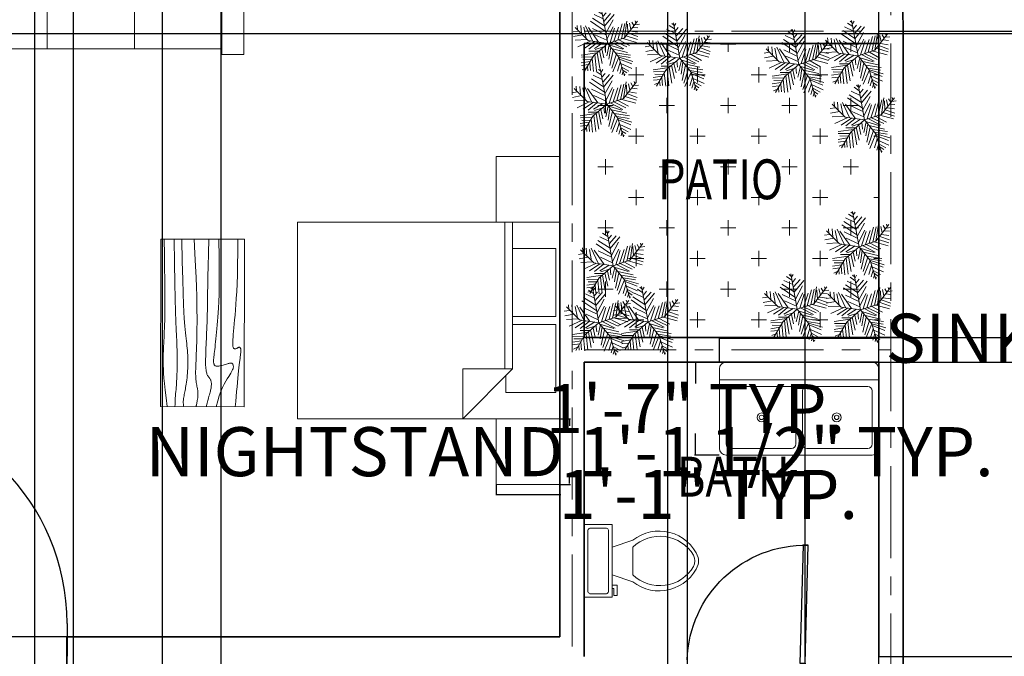
# Model space of a CAD drawing. Units: inches. Extents: x 541 to 1172, y -20 to 887.
# Tile 6 of 8: x 857 to 1058, y 588 to 717. Entities that reach past the tile are written whole.
import ezdxf

# ---------------------------------------------------------------- set-up
doc = ezdxf.new("R2010")
doc.units = ezdxf.units.IN
doc.header["$MEASUREMENT"] = 0
doc.linetypes.add('CENTER', pattern=[50.8, 31.75, -6.35, 6.35, -6.35])
doc.layers.get('0').update_dxf_attribs({"color": 70})
for name, color, linetype, lineweight in [('A-ANNO-DIMS', 2, 'Continuous', 18), ('A-AREA-IDEN', 7, 'Continuous', 20), ('A-DOOR', 4, 'Continuous', 25), ('A-FLOR-FIXT', 9, 'Continuous', 18), ('A-FURN', 30, 'Continuous', 18), ('A-WALL-CNTR', 1, 'CENTER', 13), ('L-PLNT', 70, 'Continuous', 18), ('L-PLNT-PATT', 70, 'Continuous', 13), ('WALL', 7, 'Continuous', 35)]:
    doc.layers.add(name, color=color, linetype=linetype, lineweight=lineweight)
doc.styles.get("Standard").update_dxf_attribs({"font": 'arial.ttf'})
doc.styles.add('YQ_DIM', font='SUPEROS.SHX', dxfattribs={"width": 0.8, "bigfont": 'HZDX.SHX'})
doc.dimstyles.get("Standard").update_dxf_attribs({"dimtxt": 10, "dimasz": 0.18, "dimexe": 0.18, "dimexo": 0.0625, "dimgap": 0.09, "dimtad": 0, "dimtih": 1, "dimtoh": 1, "dimdec": 1, "dimzin": 0, "dimdsep": 46, "dimlunit": 4, "dimtxsty": 'Standard', "dimcen": 0.09, "dimadec": 0, "dimazin": 0, "dimtfac": 1, "dimtdec": 1, "dimtofl": 0, "dimtmove": 0, "dimatfit": 3, "dimfxl": 1, "dimtolj": 1, "dimtzin": 0, "dimarcsym": 0})

# ---------------------------------------------------------------- blocks, each defined once
blk = doc.blocks.new('Sofa - Roundback 7 ft.')
for p, q in [((-12.00002, -32.4421), (-12.00003, -6.5971)), ((11.99997, -32.4421), (11.99998, -6.5971)), ((-36.000027, -34), (-36.000027, -11.4696)), ((-35.999844, -13.3819), (35.9998, -13.3819)), ((35.99998, -34), (35.99998, -11.4696)), ((-36.000027, -32.4421), (35.99998, -32.4421))]:
    blk.add_line(p, q)
for points in [[(-36.000027, -34), (-42.000027, -34), (-42.000027, -8)], [(41.99998, -8), (41.99998, -34), (35.99998, -34)]]:
    blk.add_lwpolyline(points)
for centre, radius, start, end in [((0, -114.25), 114.25, 68.43141, 111.5686), ((-0.00001, -127.1968), 121.1968, 72.72033, 107.2797)]:
    blk.add_arc(centre, radius, start, end)
blk = doc.blocks.new('Bed - Queen')
for p, q in [((0, -80.00003), (0, 0)), ((0, 0), (59.99999, 0)), ((59.99999, 0), (59.99999, -80.00003)), ((7.99999, -1.2), (28.79998, -1.2)), ((7.99999, -14.4), (7.99999, -1.2)), ((28.79998, -1.2), (28.79998, -14.4)), ((31.19999, -1.2), (51.99999, -1.2)), ((31.19999, -14.4), (31.19999, -1.2)), ((51.99999, -1.2), (51.99999, -16.4)), ((0, -14.4), (44.8, -14.4)), ((59.99999, -29.6), (44.8, -14.4)), ((44.8, -14.4), (44.8, -29.6)), ((44.8, -16.8), (0, -16.8)), ((51.99999, -16.4), (46.79936, -16.4)), ((44.8, -29.6), (59.99999, -29.6)), ((59.99999, -80.00003), (0, -80.00003))]:
    blk.add_line(p, q)
blk = doc.blocks.new('Table - Rectangular Woodgrain 60 x 30 in.')
for p, q in [((0, 0), (0, -30)), ((60, 0), (0, 0)), ((60, -30), (60, 0)), ((0, -30), (60, -30))]:
    blk.add_line(p, q)
for points in [[(0, -2.4), (4.8155, -2.418), (9.0302, -2.4688), (12.709, -2.5477), (15.9167, -2.65), (18.7181, -2.7711), (21.1781, -2.9063), (23.3616, -3.0508), (25.3333, -3.2), (27.1477, -3.3495), (28.8172, -3.4958), (30.3437, -3.636), (31.7291, -3.7667), (32.9756, -3.8849), (34.0849, -3.9875), (35.059, -4.0714), (35.9, -4.1334), (36.6114, -4.1711), (37.2041, -4.1854), (37.6906, -4.1779), (38.0833, -4.15), (38.3948, -4.1034), (38.6375, -4.0396), (38.8239, -3.9602), (38.9666, -3.8667), (39.0764, -3.7608), (39.1573, -3.6448), (39.2116, -3.521), (39.2416, -3.3917), (39.2498, -3.2593), (39.2385, -3.1261), (39.21, -2.9944), (39.1666, -2.8667), (39.111, -2.7447), (39.0468, -2.6281), (38.978, -2.5163), (38.9083, -2.4083), (38.8418, -2.3035), (38.7823, -2.201), (38.7337, -2.1001), (38.7, -2), (38.6844, -1.9003), (38.6875, -1.8021), (38.7094, -1.707), (38.75, -1.6167), (38.8094, -1.5326), (38.8875, -1.4563), (38.9844, -1.3893), (39.1, -1.3333), (39.2351, -1.2896), (39.3937, -1.2583), (39.5804, -1.2396), (39.8, -1.2333), (40.057, -1.2396), (40.3562, -1.2583), (40.7023, -1.2896), (41.1, -1.3333), (41.5547, -1.3895), (42.0755, -1.4573), (42.6721, -1.5361), (43.3542, -1.625), (44.1316, -1.7233), (45.014, -1.8302), (46.0114, -1.9449), (47.1333, -2.0667), (48.3862, -2.1947), (49.7625, -2.3281), (51.2513, -2.4663), (52.8416, -2.6083), (54.5226, -2.7535), (56.2833, -2.9011), (58.1127, -3.0501), (60, -3.2)], [(0, -9.2), (6.5759, -9.0858), (11.9385, -9.0365), (16.2527, -9.0418), (19.6833, -9.0917), (22.3952, -9.1759), (24.5531, -9.2844), (26.322, -9.4069), (27.8666, -9.5333), (29.3241, -9.6553), (30.7203, -9.7719), (32.0532, -9.8837), (33.3208, -9.9917), (34.5213, -10.0965), (35.6526, -10.199), (36.7128, -10.2999), (37.7, -10.4), (38.6129, -10.4996), (39.4531, -10.5969), (40.223, -10.6895), (40.925, -10.775), (41.5613, -10.8512), (42.1344, -10.9156), (42.6465, -10.966), (43.1, -11), (43.4976, -11.0158), (43.8437, -11.0136), (44.143, -10.9942), (44.4, -10.9583), (44.6195, -10.9069), (44.8062, -10.8406), (44.9648, -10.7603), (45.1, -10.6667), (45.2155, -10.5598), (45.3114, -10.4365), (45.3871, -10.2929), (45.4416, -10.125), (45.4743, -9.929), (45.4844, -9.7011), (45.4709, -9.4371), (45.4333, -9.1333), (45.3716, -8.7883), (45.2896, -8.4104), (45.1919, -8.0107), (45.0833, -7.6), (44.9685, -7.1893), (44.8521, -6.7896), (44.7388, -6.4117), (44.6333, -6.0667), (44.54, -5.7628), (44.4614, -5.4979), (44.4001, -5.2675), (44.3583, -5.0667), (44.3384, -4.8909), (44.3427, -4.7354), (44.3736, -4.5956), (44.4333, -4.4667), (44.5236, -4.3453), (44.6427, -4.2333), (44.7884, -4.1339), (44.9583, -4.05), (45.1501, -3.9849), (45.3614, -3.9417), (45.59, -3.9234), (45.8333, -3.9333), (46.0915, -3.9749), (46.3734, -4.0531), (46.6906, -4.1736), (47.0542, -4.3417), (47.4756, -4.5629), (47.9661, -4.8427), (48.5372, -5.1866), (49.2, -5.6), (49.9676, -6.0844), (50.8594, -6.625), (51.8965, -7.2031), (53.1, -7.8), (54.491, -8.3969), (56.0906, -8.975), (57.9199, -9.5156), (60, -10)], [(0, -12.8), (5.1847, -12.9322), (9.6213, -13.0323), (13.3963, -13.1059), (16.5958, -13.1583), (19.3063, -13.1952), (21.614, -13.2219), (23.6054, -13.2439), (25.3666, -13.2667), (26.9728, -13.2947), (28.4531, -13.3281), (29.8256, -13.3663), (31.1083, -13.4083), (32.3191, -13.4535), (33.476, -13.501), (34.597, -13.5501), (35.7, -13.6), (36.7984, -13.6497), (37.8875, -13.6979), (38.9578, -13.743), (40, -13.7833), (41.0047, -13.8174), (41.9625, -13.8438), (42.864, -13.8607), (43.7, -13.8667), (44.4631, -13.8604), (45.1552, -13.8417), (45.7801, -13.8104), (46.3416, -13.7667), (46.8439, -13.7104), (47.2906, -13.6417), (47.6858, -13.5604), (48.0333, -13.4667), (48.3375, -13.3608), (48.6042, -13.2448), (48.8396, -13.121), (49.05, -12.9917), (49.2417, -12.8593), (49.4208, -12.7261), (49.5937, -12.5944), (49.7667, -12.4667), (49.9452, -12.3451), (50.1323, -12.2313), (50.3303, -12.1268), (50.5416, -12.0333), (50.7686, -11.9524), (51.0135, -11.8854), (51.2788, -11.8341), (51.5666, -11.8), (51.8785, -11.7843), (52.2116, -11.7865), (52.562, -11.8059), (52.926, -11.8417), (53.2998, -11.8931), (53.6795, -11.9594), (54.0614, -12.0397), (54.4416, -12.1333), (54.8223, -12.2401), (55.2293, -12.3625), (55.6942, -12.5037), (56.2489, -12.6667), (56.9251, -12.8547), (57.7545, -13.0708), (58.7689, -13.3182), (60, -13.6)], [(0, -18), (5.124, -17.7273), (9.6609, -17.5057), (13.6705, -17.3303), (17.2125, -17.1958), (20.3467, -17.0973), (23.1328, -17.0297), (25.6307, -16.9878), (27.9, -16.9667), (29.9928, -16.9617), (31.9302, -16.9703), (33.7254, -16.9907), (35.3917, -17.0208), (36.9423, -17.0588), (38.3906, -17.1026), (39.7499, -17.1503), (41.0333, -17.2), (42.2519, -17.2496), (43.4073, -17.2969), (44.4986, -17.3395), (45.525, -17.375), (46.4858, -17.4012), (47.3802, -17.4156), (48.2074, -17.416), (48.9667, -17.4), (49.6583, -17.3662), (50.2872, -17.3167), (50.8595, -17.2547), (51.3812, -17.1833), (51.8584, -17.1057), (52.2971, -17.025), (52.7034, -16.9443), (53.0833, -16.8667), (53.443, -16.7951), (53.789, -16.7313), (54.128, -16.6768), (54.4666, -16.6334), (54.8115, -16.6024), (55.1693, -16.5854), (55.5465, -16.5841), (55.95, -16.6), (56.3828, -16.6337), (56.8346, -16.6823), (57.2915, -16.7418), (57.7396, -16.8084), (58.165, -16.878), (58.5539, -16.9469), (58.8924, -17.0111), (59.1666, -17.0667), (59.3679, -17.1107), (59.5078, -17.1438), (59.6032, -17.1675), (59.6708, -17.1833), (59.7275, -17.193), (59.7901, -17.1979), (59.8753, -17.1998), (60, -17.2)], [(0, -22.4), (8.0098, -22.2501), (14.4094, -22.1011), (19.4168, -21.9535), (23.25, -21.8083), (26.1269, -21.6663), (28.2656, -21.5281), (29.884, -21.3947), (31.2, -21.2667), (32.3967, -21.1448), (33.5172, -21.0292), (34.5697, -20.9198), (35.5625, -20.8167), (36.5037, -20.7198), (37.4015, -20.6292), (38.2642, -20.5448), (39.1, -20.4667), (39.9164, -20.3951), (40.7187, -20.3313), (41.5117, -20.2768), (42.3, -20.2333), (43.0883, -20.2024), (43.8812, -20.1854), (44.6836, -20.1841), (45.5, -20.2), (46.3328, -20.234), (47.1747, -20.2844), (48.0163, -20.3488), (48.8479, -20.425), (49.66, -20.5106), (50.4429, -20.6031), (51.1872, -20.7004), (51.8833, -20.8), (52.5246, -20.8999), (53.1166, -20.9995), (53.6681, -21.0983), (54.1875, -21.1958), (54.6834, -21.2919), (55.1646, -21.3859), (55.6394, -21.4777), (56.1167, -21.5667), (56.6028, -21.6515), (57.0961, -21.7266), (57.5929, -21.7852), (58.0896, -21.8208), (58.5823, -21.8268), (59.0674, -21.7964), (59.5412, -21.723), (60, -21.6)], [(0, -25.2), (8.6355, -25.0504), (15.7026, -24.9031), (21.4049, -24.7606), (25.9458, -24.625), (29.529, -24.4988), (32.3578, -24.3844), (34.6359, -24.284), (36.5667, -24.2), (38.3213, -24.1341), (39.9417, -24.0854), (41.437, -24.0523), (42.8167, -24.0333), (44.0901, -24.0268), (45.2667, -24.0313), (46.3557, -24.0451), (47.3667, -24.0667), (48.309, -24.0947), (49.1928, -24.1287), (50.0284, -24.168), (50.826, -24.2125), (51.5959, -24.2617), (52.3483, -24.3151), (53.0935, -24.3725), (53.8417, -24.4334), (54.6009, -24.497), (55.3699, -24.561), (56.1454, -24.6226), (56.9239, -24.6792), (57.7021, -24.7279), (58.4764, -24.7662), (59.2435, -24.7911), (60, -24.8)], [(0, -28.8), (5.6867, -28.6681), (10.45, -28.5698), (14.407, -28.5012), (17.675, -28.4584), (20.3711, -28.4374), (22.6125, -28.4344), (24.5164, -28.4455), (26.2, -28.4667), (27.762, -28.4947), (29.2276, -28.5281), (30.6033, -28.5663), (31.8958, -28.6084), (33.1118, -28.6535), (34.2578, -28.7011), (35.3405, -28.7501), (36.3666, -28.8), (37.3443, -28.8497), (38.288, -28.8974), (39.2137, -28.9412), (40.1375, -28.9792), (41.0753, -29.0093), (42.0432, -29.0297), (43.0572, -29.0384), (44.1333, -29.0333), (45.2936, -29.0114), (46.5843, -28.9641), (48.0579, -28.8816), (49.7666, -28.7542), (51.7629, -28.5721), (54.0989, -28.3255), (56.8272, -28.0048), (60, -27.6)]]:
    blk.add_lwpolyline(points)
blk = doc.blocks.new('*U7')
for p, q in [((-8.737, 47.138), (-17.069, 52.711)), ((-10.186, 53.64), (-13.084, 55.962)), ((0, 0), (-10.5, 57)), ((-9.099, 51.782), (-6.563, 55.962)), ((-7.65, 43.423), (-2.578, 49.46)), ((-5.839, 35.992), (4.667, 48.067)), ((-3.665, 19.273), (-27.574, 35.527)), ((-5.114, 28.097), (-24.676, 40.636)), ((-7.288, 39.707), (-21.778, 46.673)), ((-5.114, 27.632), (10.463, 46.673)), ((-2.941, 16.486), (8.652, 37.85)), ((22.055, 7.198), (27.489, 32.277)), ((27, 9), (48, 36)), ((27.127, 9.056), (31.112, 35.992)), ((35.096, 32.741), (37.27, 22.524)), ((38.719, 34.134), (41.979, 28.561)), ((44.153, 36.456), (45.239, 32.741)), ((-47.498, 19.737), (-55.83, 18.344)), ((-31.5, 4.5), (-52.5, 25.5)), ((-48.585, 21.131), (-49.309, 29.026)), ((-43.513, 28.561), (-42.427, 15.558)), ((-38.442, 26.239), (-34.819, 7.663)), ((-35.544, 28.097), (-24.314, 3.947)), ((-14.533, 2.09), (-30.834, 25.31)), ((-24.314, 23.917), (-2.941, 13.7)), ((-1.129, 6.734), (9.014, 26.704)), ((3.942, 1.625), (11.187, 24.381)), ((10.101, 3.483), (17.708, 26.239)), ((16.259, 5.805), (23.142, 31.348)), ((31.836, 30.883), (32.561, 16.486)), ((33.285, 16.486), (48.862, 10.913)), ((36.183, 19.737), (48.137, 17.88)), ((40.53, 25.775), (48.862, 24.846)), ((43.791, 29.954), (51.036, 30.883)), ((-40.615, 13.7), (-55.105, 10.913)), ((-33.37, 6.269), (-52.207, 5.34)), ((-28.299, 3.483), (-47.86, -5.805)), ((-21.416, 3.018), (-38.079, -8.128)), ((0, 0), (-31.5, 4.5)), ((-15.982, 2.09), (-30.11, -9.521)), ((0, 0), (-22.5, -19.5)), ((-6.563, 1.161), (-21.416, -8.128)), ((-20.691, 13.7), (-1.129, 4.876)), ((0, 0), (27, 9)), ((0, 0), (18, -22.5)), ((6.478, 1.625), (26.04, -8.592)), ((11.187, 3.483), (30.749, -5.805)), ((18.07, 5.805), (35.096, -3.483)), ((24.229, 7.663), (46.688, 1.625)), ((29.662, 12.307), (48.137, 6.269)), ((-17.431, -15.094), (-42.789, -18.809)), ((-15.257, -12.772), (-30.11, -12.772)), ((-6.563, -5.805), (-19.967, -9.985)), ((-17.069, -15.094), (-12.721, -40.172)), ((-13.446, -11.378), (-8.737, -32.741)), ((-9.461, -8.592), (-6.201, -23.453)), ((-4.752, -3.483), (-3.665, -14.629)), ((2.493, -3.019), (-1.491, -20.202)), ((1.769, -2.555), (24.229, -9.521)), ((5.029, -6.27), (2.131, -25.775)), ((9.014, -11.378), (3.58, -35.992)), ((7.565, -9.056), (32.198, -14.629)), ((12.274, -15.094), (36.907, -18.809)), ((-28.299, -29.026), (-42.789, -31.348)), ((-24.314, -21.596), (-42.427, -22.06)), ((-26.849, -26.24), (-40.253, -25.775)), ((-22.5, -19.5), (-37.5, -45)), ((-29.023, -30.884), (-27.936, -43.887)), ((-25.038, -23.918), (-22.865, -45.281)), ((-20.691, -18.345), (-17.793, -44.352)), ((14.085, -16.951), (6.478, -40.172)), ((18.07, -22.524), (8.289, -45.745)), ((20.244, -30.419), (15.897, -44.816)), ((16.259, -19.738), (36.183, -22.989)), ((18, -22.5), (27, -52.5)), ((18.433, -22.524), (40.53, -29.026)), ((19.157, -25.311), (38.719, -33.206)), ((-30.834, -34.135), (-42.427, -35.528)), ((-34.457, -39.708), (-40.978, -42.494)), ((-32.646, -36.921), (-31.921, -44.352)), ((22.78, -37.85), (19.519, -48.532)), ((21.331, -32.741), (39.081, -40.636)), ((22.78, -38.314), (34.372, -44.816)), ((24.591, -45.745), (23.142, -50.854)), ((24.591, -43.423), (30.749, -47.603)), ((26.764, -49.925), (28.213, -50.854))]:
    blk.add_line(p, q)
blk = doc.blocks.new('*U23')
for p, q in [((0, 0), (0, -6)), ((40, 0), (40, -6))]:
    blk.add_line(p, q)
blk.add_lwpolyline([(0, 0), (0, 40), (1.75, 40), (1.75, 0)], close=True)
blk.add_arc((0, 0), 40, 0, 90)
blk = doc.blocks.new('*U28')
for p, q in [((9.5, -6), (9.5, -2)), ((-10, -8.5), (-8, -8.5)), ((-10, -9.5), (-10, -8.5)), ((-8, -8.5), (-8, -8)), ((-7, -8), (-7, -9.5)), ((-4, -8), (-6, -14)), ((4, -8), (6, -14)), ((-7, -9.5), (-10, -9.5)), ((4, -14), (-4, -14))]:
    blk.add_line(p, q)
blk.add_lwpolyline([(10.5, -8), (10.5, 0), (-10.5, 0), (-10.5, -8)], close=True)
for points in [[(-9.5, -2), (-9.5, -6)], [(8.5, -1), (-8.5, -1)], [(-8.5, -7), (8.5, -7)]]:
    blk.add_lwpolyline(points)
for centre, radius, start, end in [((-8.62, -1.88), 0.884, 81.8699, 188.1301), ((8.62, -1.88), 0.884, 351.8699, 98.1301), ((-8.62, -6.12), 0.884, 171.8699, 278.1301), ((8.62, -6.12), 0.884, 261.8699, 8.1301), ((3.52, -21.58), 12.17, 141.4691, 247.9714), ((4.2, -21.82), 11.33, 136.3677, 238.9468), ((-3.52, -21.58), 12.17, 292.0284, 38.5307), ((-4.2, -21.82), 11.33, 301.053, 43.6321), ((0, -27.88), 4, 245.7318, 294.2682), ((0, -29), 4, 254.8605, 285.1395)]:
    blk.add_arc(centre, radius, start, end)
blk = doc.blocks.new('Sink-double - 36 in top')
for p, q in [((-18, -4), (18, -4)), ((-0.75, -18.5), (-0.75, -6.5)), ((0.75, -6.5), (0.75, -18.5))]:
    blk.add_line(p, q)
for points in [[(-16.5, 0), (16.5, 0)], [(-18, -19.5), (-18, -1.5)], [(18, -1.5), (18, -19.5)], [(-16.5, -18.5), (-16.5, -6.5)], [(-15.5, -5.5), (-1.75, -5.5)], [(1.75, -5.5), (15.5, -5.5)], [(16.5, -6.5), (16.5, -18.5)], [(-1.75, -19.5), (-15.5, -19.5)], [(15.5, -19.5), (1.75, -19.5)], [(16.5, -21), (-16.5, -21)]]:
    blk.add_lwpolyline(points)
for centre, radius in [((-8.5, -12.5), 1), ((-8.5, -12.5), 0.5), ((8.5, -12.5), 1), ((8.5, -12.5), 0.5)]:
    blk.add_circle(centre, radius)
for centre, radius, start, end in [((-16.5, -1.5), 1.5, 90, 180), ((16.5, -1.5), 1.5, 0, 90), ((-15.5, -6.5), 1, 90, 180), ((-1.75, -6.5), 1, 0, 90), ((1.75, -6.5), 1, 90, 180), ((15.5, -6.5), 1, 0, 90), ((-16.5, -19.5), 1.5, 180, 270), ((-15.5, -18.5), 1, 180, 270), ((-1.75, -18.5), 1, 270, 0), ((1.75, -18.5), 1, 180, 270), ((15.5, -18.5), 1, 270, 0), ((16.5, -19.5), 1.5, 270, 0)]:
    blk.add_arc(centre, radius, start, end)
blk = doc.blocks.new('FURN-NIGHTSTAND')
for p, q in [((0, 13.4), (0, 0)), ((0, 0), (13, 0))]:
    blk.add_line(p, q)
blk = doc.blocks.new('*D39')
at = {"layer": 'A-ANNO-DIMS', "color": 0, "lineweight": -2, "transparency": 16777216}
for p, q in [((684.16, 735.59), (684.16, 726.62)), ((743.21, 735.59), (743.21, 726.62)), ((684.34, 726.8), (743.03, 726.8)), ((743.21, 726.8), (743.39, 726.8))]:
    blk.add_line(p, q, dxfattribs=at)
for points in [[(684.34, 726.83), (684.34, 726.77), (684.16, 726.8)], [(743.03, 726.83), (743.03, 726.77), (743.21, 726.8)]]:
    blk.add_solid(points, dxfattribs=at)
at = {"layer": 'Defpoints', "color": 0, "lineweight": -2, "transparency": 16777216}
for p in [(684.16, 735.65), (743.21, 735.65), (743.21, 726.8)]:
    blk.add_point(p, dxfattribs=at)
at = {"layer": 'A-ANNO-DIMS', "color": 0, "transparency": 16777216, "insert": (810.64, 726.8), "char_height": 10, "attachment_point": 5}
blk.add_mtext('\\A1;WINDOW 4\'-11" TYP.', dxfattribs=at)
blk = doc.blocks.new('*D45')
at = {"layer": 'A-ANNO-DIMS', "color": 0, "lineweight": -2, "transparency": 16777216}
for p, q in [((967.35, 636.09), (969.47, 636.09)), ((969.29, 635.91), (969.29, 634.65)), ((969.29, 622.87), (969.29, 624.13)), ((967.35, 622.69), (969.47, 622.69))]:
    blk.add_line(p, q, dxfattribs=at)
for points in [[(969.26, 635.91), (969.32, 635.91), (969.29, 636.09)], [(969.26, 622.87), (969.32, 622.87), (969.29, 622.69)]]:
    blk.add_solid(points, dxfattribs=at)
at = {"layer": 'Defpoints', "color": 0, "lineweight": -2, "transparency": 16777216}
for p in [(967.28, 636.09), (969.29, 636.09), (967.28, 622.69)]:
    blk.add_point(p, dxfattribs=at)
at = {"layer": 'A-ANNO-DIMS', "color": 0, "transparency": 16777216, "insert": (969.29, 629.39), "char_height": 10, "attachment_point": 5}
blk.add_mtext('\\A1;NIGHTSTAND 1\'-1 1/2" TYP.', dxfattribs=at)
blk = doc.blocks.new('*D46')
at = {"layer": 'A-ANNO-DIMS', "color": 0, "lineweight": -2, "transparency": 16777216}
for p, q in [((954.28, 622.63), (954.28, 620.5)), ((967.28, 622.63), (967.28, 620.5)), ((954.46, 620.68), (967.1, 620.68)), ((967.28, 620.68), (967.46, 620.68))]:
    blk.add_line(p, q, dxfattribs=at)
for points in [[(954.46, 620.71), (954.46, 620.65), (954.28, 620.68)], [(967.1, 620.71), (967.1, 620.65), (967.28, 620.68)]]:
    blk.add_solid(points, dxfattribs=at)
at = {"layer": 'Defpoints', "color": 0, "lineweight": -2, "transparency": 16777216}
for p in [(954.28, 622.69), (967.28, 622.69), (967.28, 620.68)]:
    blk.add_point(p, dxfattribs=at)
at = {"layer": 'A-ANNO-DIMS', "color": 0, "transparency": 16777216, "insert": (997.56, 620.68), "char_height": 10, "attachment_point": 5}
blk.add_mtext('\\A1;1\'-1" TYP.', dxfattribs=at)
blk = doc.blocks.new('*D51')
at = {"layer": 'A-ANNO-DIMS', "color": 0, "lineweight": -2, "transparency": 16777216}
for p, q in [((999.81, 647.72), (999.81, 652.71)), ((999.99, 652.53), (1032.1, 652.53)), ((1032.28, 647.72), (1032.28, 652.71)), ((1032.28, 652.53), (1032.46, 652.53))]:
    blk.add_line(p, q, dxfattribs=at)
for points in [[(999.99, 652.56), (999.99, 652.5), (999.81, 652.53)], [(1032.1, 652.56), (1032.1, 652.5), (1032.28, 652.53)]]:
    blk.add_solid(points, dxfattribs=at)
at = {"layer": 'Defpoints', "color": 0, "lineweight": -2, "transparency": 16777216}
for p in [(1032.28, 652.53), (999.81, 647.65), (1032.28, 647.65)]:
    blk.add_point(p, dxfattribs=at)
at = {"layer": 'A-ANNO-DIMS', "color": 0, "transparency": 16777216, "insert": (1092.9, 652.53), "char_height": 10, "attachment_point": 5}
blk.add_mtext('\\A1;SINK 2\'-8 1/2" TYP.', dxfattribs=at)
blk = doc.blocks.new('*D52')
at = {"layer": 'A-ANNO-DIMS', "color": 0, "lineweight": -2, "transparency": 16777216}
for p, q in [((999.75, 647.65), (994.76, 647.65)), ((994.94, 647.47), (994.94, 643.3)), ((994.94, 628.89), (994.94, 633.07)), ((999.75, 628.71), (994.76, 628.71))]:
    blk.add_line(p, q, dxfattribs=at)
for points in [[(994.91, 647.47), (994.97, 647.47), (994.94, 647.65)], [(994.91, 628.89), (994.97, 628.89), (994.94, 628.71)]]:
    blk.add_solid(points, dxfattribs=at)
at = {"layer": 'Defpoints', "color": 0, "lineweight": -2, "transparency": 16777216}
for p in [(994.94, 647.65), (999.81, 647.65), (999.81, 628.71)]:
    blk.add_point(p, dxfattribs=at)
at = {"layer": 'A-ANNO-DIMS', "color": 0, "transparency": 16777216, "insert": (994.94, 638.18), "char_height": 10, "attachment_point": 5}
blk.add_mtext('\\A1;1\'-7" TYP.', dxfattribs=at)
blk = doc.blocks.new('*D61')
at = {"layer": 'A-ANNO-DIMS', "color": 0, "lineweight": -2, "transparency": 16777216}
for p, q in [((802.49, 574.25), (802.49, 579.28)), ((802.67, 579.1), (835.09, 579.1)), ((835.27, 574.25), (835.27, 579.28)), ((835.27, 579.1), (835.45, 579.1))]:
    blk.add_line(p, q, dxfattribs=at)
for points in [[(802.67, 579.13), (802.67, 579.07), (802.49, 579.1)], [(835.09, 579.13), (835.09, 579.07), (835.27, 579.1)]]:
    blk.add_solid(points, dxfattribs=at)
at = {"layer": 'Defpoints', "color": 0, "lineweight": -2, "transparency": 16777216}
for p in [(835.27, 579.1), (802.49, 574.19), (835.27, 574.19)]:
    blk.add_point(p, dxfattribs=at)
at = {"layer": 'A-ANNO-DIMS', "color": 0, "transparency": 16777216, "insert": (896.96, 579.1), "char_height": 10, "attachment_point": 5}
blk.add_mtext('\\A1;ACCENT 2\'-9" TYP.', dxfattribs=at)
blk = doc.blocks.new('*D70')
at = {"layer": 'A-ANNO-DIMS', "color": 0, "lineweight": -2, "transparency": 16777216}
for p, q in [((1036.7, 829.68), (1143.21, 829.68)), ((1143.03, 829.5), (1143.03, 444.36)), ((1143.03, 48.83), (1143.03, 433.97)), ((1037.35, 48.65), (1143.21, 48.65))]:
    blk.add_line(p, q, dxfattribs=at)
for points in [[(1143, 829.5), (1143.06, 829.5), (1143.03, 829.68)], [(1143, 48.83), (1143.06, 48.83), (1143.03, 48.65)]]:
    blk.add_solid(points, dxfattribs=at)
at = {"layer": 'Defpoints', "color": 0, "lineweight": -2, "transparency": 16777216}
for p in [(1036.64, 829.68), (1037.28, 48.65), (1143.03, 48.65)]:
    blk.add_point(p, dxfattribs=at)
at = {"layer": 'A-ANNO-DIMS', "color": 0, "transparency": 16777216, "insert": (1143.03, 439.17), "char_height": 10, "attachment_point": 5}
blk.add_mtext('\\A1;65\'-1"', dxfattribs=at)
blk = doc.blocks.new('*D80')
at = {"layer": 'A-ANNO-DIMS', "color": 0, "lineweight": -2, "transparency": 16777216}
for p, q in [((1032.33, 715.15), (1143.21, 715.15)), ((1143.03, 714.97), (1143.03, 689.16)), ((1143.03, 652.83), (1143.03, 678.64)), ((1032.35, 652.65), (1143.21, 652.65))]:
    blk.add_line(p, q, dxfattribs=at)
for points in [[(1143, 714.97), (1143.06, 714.97), (1143.03, 715.15)], [(1143, 652.83), (1143.06, 652.83), (1143.03, 652.65)]]:
    blk.add_solid(points, dxfattribs=at)
at = {"layer": 'Defpoints', "color": 0, "lineweight": -2, "transparency": 16777216}
for p in [(1032.27, 715.15), (1032.28, 652.65), (1143.03, 652.65)]:
    blk.add_point(p, dxfattribs=at)
at = {"layer": 'A-ANNO-DIMS', "color": 0, "transparency": 16777216, "insert": (1143.03, 683.9), "char_height": 10, "attachment_point": 5}
blk.add_mtext('\\A1;5\'-2 1/2"', dxfattribs=at)
blk = doc.blocks.new('*D81')
at = {"layer": 'A-ANNO-DIMS', "color": 0, "lineweight": -2, "transparency": 16777216}
for p, q in [((1032.35, 647.65), (1143.21, 647.65)), ((1143.03, 647.47), (1143.03, 622.85)), ((1143.03, 587.83), (1143.03, 612.46)), ((1032.35, 587.65), (1143.21, 587.65))]:
    blk.add_line(p, q, dxfattribs=at)
for points in [[(1143, 647.47), (1143.06, 647.47), (1143.03, 647.65)], [(1143, 587.83), (1143.06, 587.83), (1143.03, 587.65)]]:
    blk.add_solid(points, dxfattribs=at)
at = {"layer": 'Defpoints', "color": 0, "lineweight": -2, "transparency": 16777216}
for p in [(1032.28, 647.65), (1032.28, 587.65), (1143.03, 587.65)]:
    blk.add_point(p, dxfattribs=at)
at = {"layer": 'A-ANNO-DIMS', "color": 0, "transparency": 16777216, "insert": (1143.03, 617.65), "char_height": 10, "attachment_point": 5}
blk.add_mtext('\\A1;5\'-0"', dxfattribs=at)
blk = doc.blocks.new('*D89')
at = {"layer": 'A-ANNO-DIMS', "color": 0, "lineweight": -2, "transparency": 16777216}
for p, q in [((989.28, 430.72), (989.28, 872.66)), ((989.46, 872.48), (997.41, 872.48)), ((1032.1, 872.48), (1024.16, 872.48)), ((1032.28, 430.72), (1032.28, 872.66))]:
    blk.add_line(p, q, dxfattribs=at)
for points in [[(989.46, 872.51), (989.46, 872.45), (989.28, 872.48)], [(1032.1, 872.51), (1032.1, 872.45), (1032.28, 872.48)]]:
    blk.add_solid(points, dxfattribs=at)
at = {"layer": 'Defpoints', "color": 0, "lineweight": -2, "transparency": 16777216}
for p in [(1032.28, 872.48), (989.28, 430.65), (1032.28, 430.65)]:
    blk.add_point(p, dxfattribs=at)
at = {"layer": 'A-ANNO-DIMS', "color": 0, "transparency": 16777216, "insert": (1010.78, 872.48), "char_height": 10, "attachment_point": 5}
blk.add_mtext('\\A1;3\'-7"', dxfattribs=at)
blk = doc.blocks.new('*D97')
at = {"layer": 'A-ANNO-DIMS', "color": 0, "lineweight": -2, "transparency": 16777216}
for p, q in [((886.28, 430.72), (886.28, 872.66)), ((886.46, 872.48), (898.1, 872.48)), ((898.28, 430.72), (898.28, 872.66)), ((898.28, 872.48), (898.46, 872.48))]:
    blk.add_line(p, q, dxfattribs=at)
for points in [[(886.46, 872.51), (886.46, 872.45), (886.28, 872.48)], [(898.1, 872.51), (898.1, 872.45), (898.28, 872.48)]]:
    blk.add_solid(points, dxfattribs=at)
at = {"layer": 'Defpoints', "color": 0, "lineweight": -2, "transparency": 16777216}
for p in [(898.28, 872.48), (886.28, 430.65), (898.28, 430.65)]:
    blk.add_point(p, dxfattribs=at)
at = {"layer": 'A-ANNO-DIMS', "color": 0, "transparency": 16777216, "insert": (911.37, 872.48), "char_height": 10, "attachment_point": 5}
blk.add_mtext('\\A1;1\'-0"', dxfattribs=at)
blk = doc.blocks.new('*D98')
at = {"layer": 'A-ANNO-DIMS', "color": 0, "lineweight": -2, "transparency": 16777216}
for p, q in [((993.28, 326.72), (993.28, 872.66)), ((993.46, 872.48), (1017.14, 872.48)), ((1017.32, 326.72), (1017.32, 872.66)), ((1017.32, 872.48), (1017.5, 872.48))]:
    blk.add_line(p, q, dxfattribs=at)
for points in [[(993.46, 872.51), (993.46, 872.45), (993.28, 872.48)], [(1017.14, 872.51), (1017.14, 872.45), (1017.32, 872.48)]]:
    blk.add_solid(points, dxfattribs=at)
at = {"layer": 'Defpoints', "color": 0, "lineweight": -2, "transparency": 16777216}
for p in [(1017.32, 872.48), (993.28, 326.65), (1017.32, 326.65)]:
    blk.add_point(p, dxfattribs=at)
at = {"layer": 'A-ANNO-DIMS', "color": 0, "transparency": 16777216, "insert": (1030.97, 872.48), "char_height": 10, "attachment_point": 5}
blk.add_mtext('\\A1;2\'-0"', dxfattribs=at)
blk = doc.blocks.new('*D101')
at = {"layer": 'A-ANNO-DIMS', "color": 0, "lineweight": -2, "transparency": 16777216}
for p, q in [((805.35, 735.65), (1143.21, 735.65)), ((1143.03, 735.47), (1143.03, 730.35)), ((1143.03, 714.83), (1143.03, 719.96)), ((805.35, 714.65), (1143.21, 714.65))]:
    blk.add_line(p, q, dxfattribs=at)
for points in [[(1143, 735.47), (1143.06, 735.47), (1143.03, 735.65)], [(1143, 714.83), (1143.06, 714.83), (1143.03, 714.65)]]:
    blk.add_solid(points, dxfattribs=at)
at = {"layer": 'Defpoints', "color": 0, "lineweight": -2, "transparency": 16777216}
for p in [(805.28, 735.65), (1143.03, 735.65), (805.28, 714.65)]:
    blk.add_point(p, dxfattribs=at)
at = {"layer": 'A-ANNO-DIMS', "color": 0, "transparency": 16777216, "insert": (1143.03, 725.15), "char_height": 10, "attachment_point": 5}
blk.add_mtext('\\A1;1\'-9"', dxfattribs=at)
blk = doc.blocks.new('*D104')
at = {"layer": 'A-ANNO-DIMS', "color": 0, "lineweight": -2, "transparency": 16777216}
for p, q in [((860.28, 177.72), (860.28, 872.66)), ((860.46, 872.48), (867.98, 872.48)), ((868.16, 177.72), (868.16, 872.66)), ((868.16, 872.48), (868.34, 872.48))]:
    blk.add_line(p, q, dxfattribs=at)
for points in [[(860.46, 872.51), (860.46, 872.45), (860.28, 872.48)], [(867.98, 872.51), (867.98, 872.45), (868.16, 872.48)]]:
    blk.add_solid(points, dxfattribs=at)
at = {"layer": 'Defpoints', "color": 0, "lineweight": -2, "transparency": 16777216}
for p in [(868.16, 872.48), (860.28, 177.65), (868.16, 177.65)]:
    blk.add_point(p, dxfattribs=at)
at = {"layer": 'A-ANNO-DIMS', "color": 0, "transparency": 16777216, "insert": (881.72, 872.48), "char_height": 10, "attachment_point": 5}
blk.add_mtext('\\A1;0\'-8"', dxfattribs=at)
blk = doc.blocks.new('*D107')
at = {"layer": 'A-ANNO-DIMS', "color": 0, "lineweight": -2, "transparency": 16777216}
for p, q in [((967.22, 735.65), (573.66, 735.65)), ((573.84, 735.47), (573.84, 668.85)), ((573.84, 591.83), (573.84, 658.46)), ((967.22, 591.65), (573.66, 591.65))]:
    blk.add_line(p, q, dxfattribs=at)
for points in [[(573.81, 735.47), (573.87, 735.47), (573.84, 735.65)], [(573.81, 591.83), (573.87, 591.83), (573.84, 591.65)]]:
    blk.add_solid(points, dxfattribs=at)
at = {"layer": 'Defpoints', "color": 0, "lineweight": -2, "transparency": 16777216}
for p in [(967.28, 735.65), (573.84, 591.65), (967.28, 591.65)]:
    blk.add_point(p, dxfattribs=at)
at = {"layer": 'A-ANNO-DIMS', "color": 0, "transparency": 16777216, "insert": (573.84, 663.65), "char_height": 10, "attachment_point": 5}
blk.add_mtext('\\A1;12\'-0"', dxfattribs=at)

msp = doc.modelspace()

# ---------------------------------------------------------------- hatches: boundary and pattern name
at = {"layer": 'L-PLNT-PATT'}
h = msp.add_hatch(dxfattribs=at)
h.set_pattern_fill('CROSS', color=256, scale=25)
h.paths.add_polyline_path([(972.28, 652.65), (1032.28, 652.65), (1032.28, 712.65), (972.28, 712.65)])

# ---------------------------------------------------------------- linework, layer by layer
at = {"layer": 'A-WALL-CNTR', "ltscale": 0.590551}
for p, q in [((1034.15, 827.18), (1034.77, 715.15)), ((969.78, 589.65), (969.78, 738.15)), ((972.28, 715.15), (1032.27, 715.15)), ((1034.78, 247.65), (1034.78, 712.65)), ((972.28, 650.15), (1034.78, 650.15))]:
    msp.add_line(p, q, dxfattribs=at)
at = {"layer": 'WALL'}
for p, q in [((1036.64, 829.68), (1037.28, 712.65)), ((967.28, 735.65), (967.28, 712.65)), ((967.28, 591.65), (967.28, 712.65)), ((972.28, 712.65), (1032.28, 712.65)), ((972.28, 652.65), (972.28, 712.65)), ((1032.28, 652.65), (1032.28, 712.65)), ((1037.28, 48.65), (1037.28, 712.65)), ((972.28, 652.65), (1037.28, 652.65)), ((972.28, 647.65), (1032.28, 647.65)), ((972.28, 587.65), (972.28, 647.65)), ((1032.28, 587.65), (1032.28, 647.65)), ((866.83, 591.65), (866.83, 582.65)), ((866.83, 591.65), (967.28, 591.65))]:
    msp.add_line(p, q, dxfattribs=at)

# ---------------------------------------------------------------- block references
at = {"layer": 'A-DOOR', "xscale": 1.115231810502029, "yscale": 1.115231810502029, "zscale": 1.115231810502029}
msp.add_blockref('*U23', (822.26, 594.38), dxfattribs=at)
at = {"layer": 'A-DOOR', "xscale": -0.6011813567709343, "yscale": 0.6011813567709343, "zscale": 0.6011813567709343, "rotation": 358.4510988302025}
msp.add_blockref('*U23', (1017.28, 586.26), dxfattribs=at)
at = {"layer": 'A-FLOR-FIXT', "xscale": 0.9019743609965102, "yscale": 0.9019743609965102, "zscale": 0.9019743609965102}
msp.add_blockref('Sink-double - 36 in top', (1016.05, 647.65), dxfattribs=at)
at = {"layer": 'A-FLOR-FIXT', "xscale": 0.7059824596600022, "yscale": 0.7059824596600022, "zscale": 0.7059824596600022, "rotation": 90.00000000000043}
msp.add_blockref('*U28', (972.28, 607.1), dxfattribs=at)
at = {"layer": 'A-FURN', "xscale": 0.7424226432878923, "yscale": 0.7424226432878923, "zscale": 0.7424226432878923}
msp.add_blockref('Sofa - Roundback 7 ft.', (871.71, 735.65), dxfattribs=at)
at = {"layer": 'A-FURN', "extrusion": (0, 0, -1), "zscale": -1, "rotation": 180}
msp.add_blockref('FURN-NIGHTSTAND', (-954.28, 689.6), dxfattribs=at)
at = {"layer": 'A-FURN'}
for name, p, xscale, yscale, zscale, rotation in [('Bed - Queen', (967.28, 676.2), 0.6685054037368693, 0.6685054037368693, 0.6685054037368693, 270), ('Table - Rectangular Woodgrain 60 x 30 in.', (903.03, 672.71), 0.5694163205475999, 0.5694163205475999, 0.5694163205475999, 269.908106286482)]:
    msp.add_blockref(name, p, dxfattribs=dict(at, xscale=xscale, yscale=yscale, zscale=zscale, rotation=rotation))
msp.add_blockref('FURN-NIGHTSTAND', (954.28, 622.7), dxfattribs=at)
at = {"layer": 'L-PLNT', "xscale": 0.1264207715891114, "yscale": 0.1264207715891114, "zscale": 0.1264207715891114}
for p in [(977.04, 712.66), (991.75, 709.63), (1028.09, 710.11), (1015.99, 708.34), (976.85, 700.26), (1029.41, 697.03), (1028.28, 671.19), (978.17, 667.31), (1015.67, 658.43), (1028.6, 658.29), (975.26, 655.69), (985.28, 655.84)]:
    msp.add_blockref('*U7', p, dxfattribs=at)

# ---------------------------------------------------------------- texts
at = {"layer": 'A-AREA-IDEN', "style": 'YQ_DIM', "width": 0.8}
for s, p in [(' PATIO', (985.31, 680.87)), ('BATH', (991.14, 620.22))]:
    msp.add_text(s, height=8.13, dxfattribs=at).set_placement(p)

# ---------------------------------------------------------------- dimensions: what is measured, and where the dimension line sits
at = {"layer": 'A-ANNO-DIMS'}
for base, p1, p2, picture, middle in [((868.16, 872.48), (860.28, 177.65), (868.16, 177.65), '*D104', (881.72, 872.48)), ((898.28, 872.48), (886.28, 430.65), (898.28, 430.65), '*D97', (911.37, 872.48)), ((1032.28, 872.48), (989.28, 430.65), (1032.28, 430.65), '*D89', (1010.78, 872.48)), ((1017.32, 872.48), (993.28, 326.65), (1017.32, 326.65), '*D98', (1030.97, 872.48))]:
    dim = msp.add_linear_dim(base=base, p1=p1, p2=p2, dimstyle='Standard', override={"dimdec": 1, "dimlfac": 1, "dimrnd": 0, "dimzin": 1, "dimdsep": 46, "dimlunit": 4, "dimfrac": 2}, dxfattribs=at)
    dim.commit()
    dim.dimension.update_dxf_attribs({"geometry": picture, "text_midpoint": middle})
for base, p1, p2, picture, middle in [((1143.03, 48.65), (1036.64, 829.68), (1037.28, 48.65), '*D70', (1143.03, 439.17)), ((573.84, 591.65), (967.28, 735.65), (967.28, 591.65), '*D107', (573.84, 663.65)), ((1143.03, 735.65), (805.28, 714.65), (805.28, 735.65), '*D101', (1143.03, 725.15)), ((1143.03, 652.65), (1032.27, 715.15), (1032.28, 652.65), '*D80', (1143.03, 683.9)), ((1143.03, 587.65), (1032.28, 647.65), (1032.28, 587.65), '*D81', (1143.03, 617.65))]:
    dim = msp.add_linear_dim(base=base, p1=p1, p2=p2, angle=90, dimstyle='Standard', override={"dimdec": 1, "dimlfac": 1, "dimrnd": 0, "dimzin": 1, "dimdsep": 46, "dimlunit": 4, "dimfrac": 2}, dxfattribs=at)
    dim.commit()
    dim.dimension.update_dxf_attribs({"geometry": picture, "text_midpoint": middle})
for base, p1, p2, text, picture, middle in [((743.2125, 726.7962), (684.1574, 735.6544), (743.2125, 735.6544), 'WINDOW <> TYP.', '*D39', (810.638, 726.7962)), ((1032.28, 652.53), (999.81, 647.65), (1032.28, 647.65), 'SINK <> TYP.', '*D51', (1092.9, 652.53)), ((967.28, 620.68), (954.28, 622.69), (967.28, 622.69), '<> TYP.', '*D46', (997.56, 620.68)), ((835.27, 579.1), (802.49, 574.19), (835.27, 574.19), 'ACCENT <> TYP.', '*D61', (896.96, 579.1))]:
    dim = msp.add_linear_dim(base=base, p1=p1, p2=p2, text=text, dimstyle='Standard', override={"dimdec": 1, "dimlfac": 1, "dimrnd": 0, "dimzin": 1, "dimdsep": 46, "dimlunit": 4, "dimfrac": 2}, dxfattribs=at)
    dim.commit()
    dim.dimension.update_dxf_attribs({"geometry": picture, "text_midpoint": middle})
for base, p1, p2, text, picture, middle in [((969.29, 636.09), (967.28, 622.69), (967.28, 636.09), 'NIGHTSTAND <> TYP.', '*D45', (969.29, 629.39)), ((994.94, 647.65), (999.81, 628.71), (999.81, 647.65), '<> TYP.', '*D52', (994.94, 638.18))]:
    dim = msp.add_linear_dim(base=base, p1=p1, p2=p2, angle=90, text=text, dimstyle='Standard', override={"dimdec": 1, "dimlfac": 1, "dimrnd": 0, "dimzin": 1, "dimdsep": 46, "dimlunit": 4, "dimfrac": 2}, dxfattribs=at)
    dim.commit()
    dim.dimension.update_dxf_attribs({"geometry": picture, "text_midpoint": middle})

doc.saveas('drawing.dxf')
